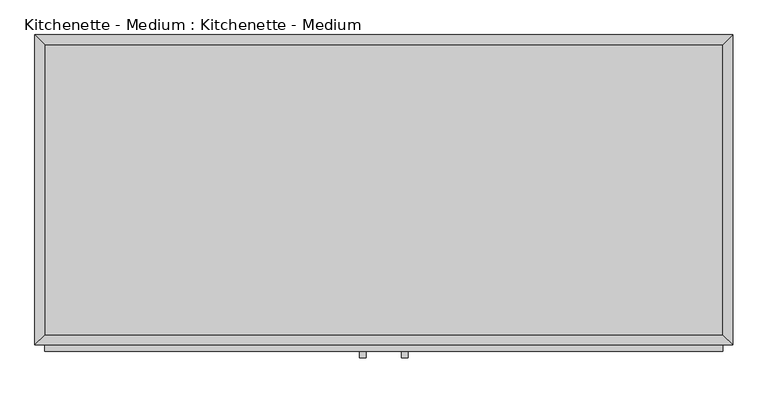
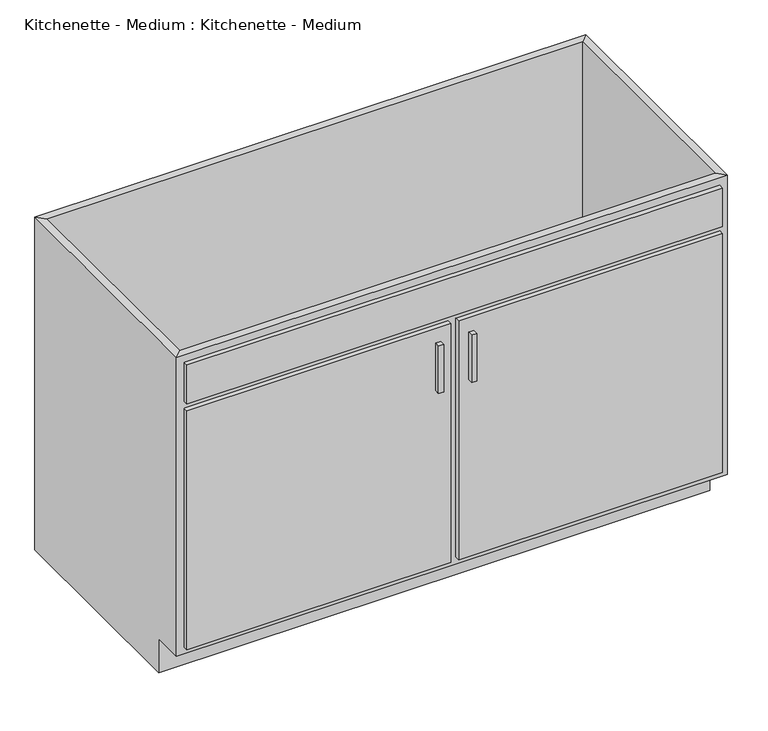
"""IFC4 building model written with IfcOpenShell, lengths in millimetres: proxy geometry, Kitchenette - Medium : Kitchenette - Medium."""

from ifc_helpers import new_model, si_unit, frame, origin, place, context, project, spatial, polyline, outline, extrude, faceted_brep, source, transform, mapped, element, save


def kitchenette_medium_kitchenette_medium_844211aa(model_context):
    return source(origin(), model_context, "Body", "SolidModel", [
        faceted_brep([(685.4877049, -590.55, 876.3), (685.4877049, -590.55, 88.9), (-648.0122951, -590.55, 88.9), (-648.0122951, -590.55, 876.3), (-667.0622951, -609.6, 876.3), (704.5377049, -609.6, 876.3), (-667.0622951, -609.6, 88.9), (704.5377049, -609.6, 88.9), (-648.0122951, -533.4, 88.9), (-648.0122951, -19.05, 88.9), (-648.0122951, -19.05, 876.3), (-667.0622951, 0.0, 876.3), (-667.0622951, 0.0, 0.0), (-667.0622951, -533.4, 0.0), (-667.0622951, -533.4, 88.9), (685.4877049, -19.05, 88.9), (685.4877049, -19.05, 876.3), (704.5377049, 0.0, 876.3), (704.5377049, 0.0, 0.0), (685.4877049, -533.4, 88.9), (704.5377049, -533.4, 88.9), (704.5377049, -533.4, 0.0)], [[[0, 1, 2, 3]], [[0, 3, 4, 5]], [[5, 4, 6, 7]], [[2, 1, 7, 6]], [[3, 2, 8, 9, 10]], [[4, 3, 10, 11]], [[6, 4, 11, 12, 13, 14]], [[2, 6, 14, 8]], [[10, 9, 15, 16]], [[11, 10, 16, 17]], [[12, 11, 17, 18]], [[1, 0, 16, 15, 19]], [[0, 5, 17, 16]], [[5, 7, 20, 21, 18, 17]], [[7, 1, 19, 20]], [[8, 19, 15, 9]], [[18, 21, 13, 12]], [[13, 21, 20, 19, 8, 14]]]),
        extrude(outline(polyline([(-16.1872951, -635.0), (-28.8872951, -635.0), (-28.8872951, -622.3), (-16.1872951, -622.3), (-16.1872951, -635.0)])), frame((0.0, 0.0, 573.769895), z_axis=(0.0, 0.0, 1.0), x_axis=(1.0, 0.0, 0.0)), (0.0, 0.0, 1.0), 124.730105),
        extrude(outline(polyline([(66.3627049, -635.0), (53.6627049, -635.0), (53.6627049, -622.3), (66.3627049, -622.3), (66.3627049, -635.0)])), frame((0.0, 0.0, 573.769895), z_axis=(0.0, 0.0, 1.0), x_axis=(1.0, 0.0, 0.0)), (0.0, 0.0, 1.0), 124.730105),
        extrude(outline(polyline([(685.4877049, -19.05), (685.4877049, -590.55), (-648.0122951, -590.55), (-648.0122951, -19.05), (685.4877049, -19.05)])), frame((0.0, 0.0, 88.9), z_axis=(0.0, 0.0, 1.0), x_axis=(1.0, 0.0, 0.0)), (0.0, 0.0, 1.0), 19.05),
        extrude(outline(polyline([(9.2127049, -622.3), (-648.0122951, -622.3), (-648.0122951, -609.6), (9.2127049, -609.6), (9.2127049, -622.3)])), frame((0.0, 0.0, 107.95), z_axis=(0.0, 0.0, 1.0), x_axis=(1.0, 0.0, 0.0)), (0.0, 0.0, 1.0), 628.65),
        extrude(outline(polyline([(685.4877049, -622.3), (28.2627049, -622.3), (28.2627049, -609.6), (685.4877049, -609.6), (685.4877049, -622.3)])), frame((0.0, 0.0, 107.95), z_axis=(0.0, 0.0, 1.0), x_axis=(1.0, 0.0, 0.0)), (0.0, 0.0, 1.0), 628.65),
        extrude(outline(polyline([(685.4877049, -622.3), (-648.0122951, -622.3), (-648.0122951, -609.6), (685.4877049, -609.6), (685.4877049, -622.3)])), frame((0.0, 0.0, 755.65), z_axis=(0.0, 0.0, 1.0), x_axis=(1.0, 0.0, 0.0)), (0.0, 0.0, 1.0), 101.6),
    ])


if __name__ == "__main__":
    model = new_model("IFC4")
    model_context = context("Model", 3, world=origin())
    ifc_project = project(units=[si_unit("LENGTHUNIT", "METRE", prefix="MILLI")], contexts=[model_context])
    site = spatial("IfcSite", under=ifc_project)
    building = spatial("IfcBuilding", under=site)
    placement = place(None, origin())
    kitchenette_medium_kitchenette_medium_shape = kitchenette_medium_kitchenette_medium_844211aa(model_context)
    element("IfcBuildingElementProxy", 1, Name="Kitchenette - Medium : Kitchenette - Medium", ObjectType="Kitchenette - Medium : Kitchenette - Medium", at=placement, inside=building, context=model_context, shape_type="MappedRepresentation", body=[
        mapped(kitchenette_medium_kitchenette_medium_shape, transform((0.0, 0.0, 0.0), x_axis=(1.0, 0.0, 0.0), y_axis=(0.0, 1.0, 0.0), z_axis=(0.0, 0.0, 1.0))),
    ])
    save(model, "model.ifc")

# Revit data of these elements
# Type "Kitchenette - Medium : Kitchenette - Medium"
#   Assembly Code = "E1090400"
#   Counter Length = 5' - 6"
#   Cabinet Width = 4' - 6"
#   Cabinet Height = 2' - 10 1/2"
#   Cabinet Depth = 2' - 0"
#   Toe Depth = 0' - 3"
#   Toe Height = 0' - 3 1/2"
#   Cabinet Material = Cabinets
#   Door/Drawer Material = Cabinets
#   Handle Material = Cabinets - Handles
#   Default Elevation = 0
# Element 1 (IfcBuildingElementProxy, "Kitchenette - Medium : Kitchenette - Medium")
#   Materials on its faces: "Cabinets", "Cabinets - Handles"
# Materials
#   "Cabinets": colour RGB 249 249 249, transparency 0
#   "Cabinets - Handles": class "Metal", colour RGB 57 57 57, transparency 0
